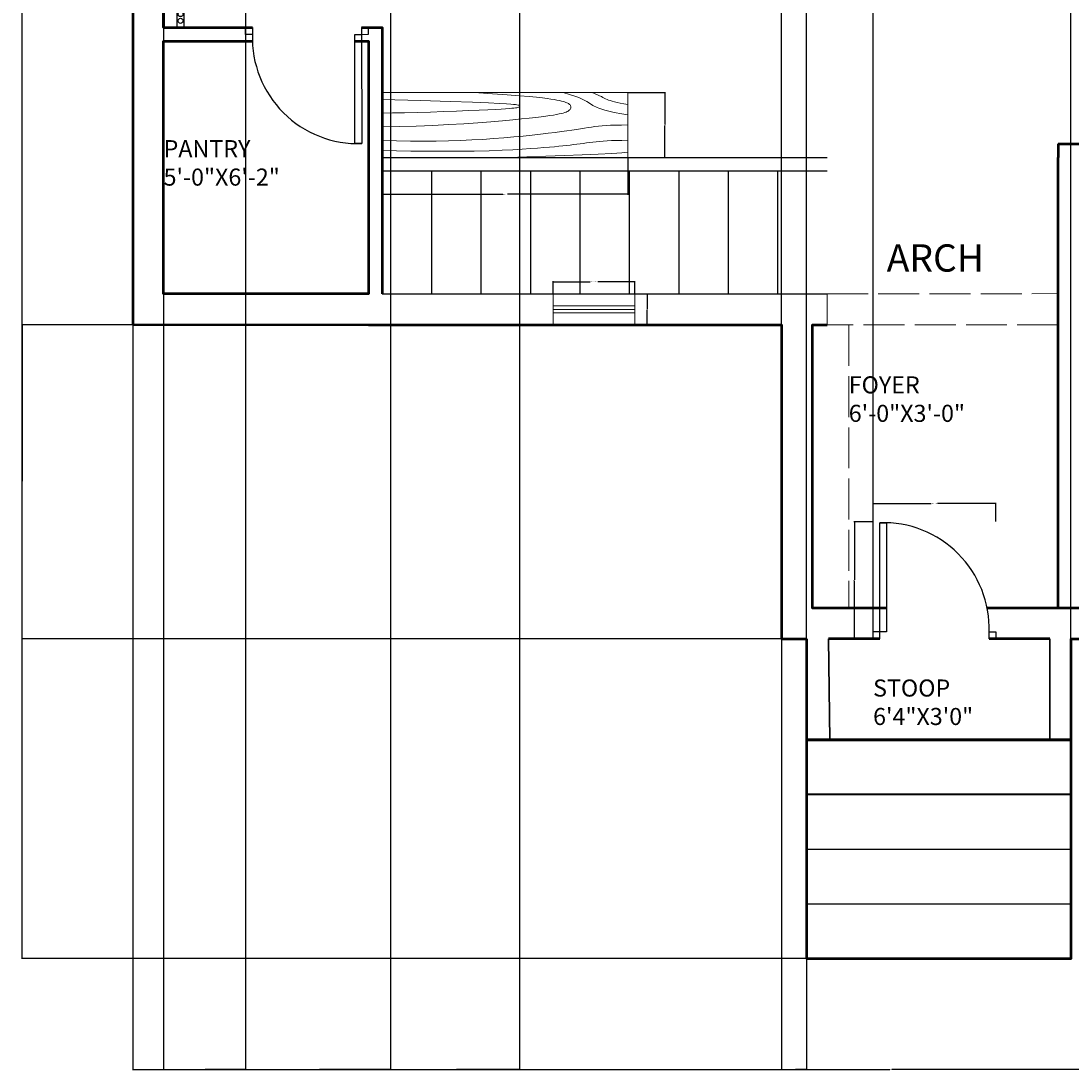
# Model space of a CAD drawing. Units: inches. Extents: x 821 to 2399, y 74 to 823.
# Tile 1 of 13: x 821 to 1128, y 74 to 381. Entities that reach past the tile are written whole.
import ezdxf

# ---------------------------------------------------------------- set-up
doc = ezdxf.new("R2010")
doc.units = ezdxf.units.IN
doc.header["$MEASUREMENT"] = 0
doc.linetypes.add('ACAD_ISO02W100', pattern=[15, 12, -3])
doc.layers.get('0').update_dxf_attribs({"lineweight": 53})
for name, color, linetype, lineweight in [('A-ANNO-DIMS', 2, 'Continuous', 18), ('A-ANNO-TEXT', 7, 'Continuous', 18), ('A-AREA-IDEN', 7, 'Continuous', 18), ('A-DOOR', 4, 'Continuous', 25), ('A-EQPM', 9, 'Continuous', 25), ('A-FLOR', 7, 'Continuous', 30), ('A-FLOR-CASE', 9, 'Continuous', 25), ('A-FLOR-STRS', 7, 'Continuous', 25), ('A-FURN', 8, 'Continuous', 18), ('A-GLAZ', 4, 'Continuous', 18), ('A-WALL-OVHD', 8, 'ACAD_ISO02W100', 18), ('WALLS', 7, 'Continuous', 50)]:
    doc.layers.add(name, color=color, linetype=linetype, lineweight=lineweight)
doc.styles.get("Standard").update_dxf_attribs({"font": 'arial.ttf'})
doc.dimstyles.get("Standard").update_dxf_attribs({"dimtxt": 0.18, "dimasz": 0.18, "dimexe": 0.18, "dimexo": 0.0625, "dimgap": 0.09, "dimtad": 0, "dimtih": 1, "dimtoh": 1, "dimdec": 4, "dimzin": 0, "dimdsep": 46, "dimtxsty": 'Standard', "dimcen": 0.09, "dimadec": 0, "dimazin": 0, "dimtfac": 1, "dimtdec": 4, "dimtofl": 0, "dimtmove": 0, "dimatfit": 3, "dimfxl": 1, "dimtolj": 1, "dimtzin": 0, "dimarcsym": 0})

# ---------------------------------------------------------------- blocks, each defined once
blk = doc.blocks.new('Hutch - 19 x 72 in.')
for p, q in [((0, -19), (0, 0)), ((0, 0), (71.999994, 0)), ((71.999994, 0), (71.999994, -19)), ((71.999994, -19), (0, -19))]:
    blk.add_line(p, q)
for points in [[(26.99999, 0), (32.30411, -0.35238), (36.66731, -0.66276), (40.20336, -0.93603), (43.02603, -1.17708), (45.2491, -1.39079), (46.98632, -1.58203), (48.35147, -1.7557), (49.45833, -1.91667), (50.40388, -2.06917), (51.21809, -2.21484), (51.91414, -2.35465), (52.5052, -2.48958), (53.00447, -2.6206), (53.42512, -2.7487), (53.78035, -2.87484), (54.08333, -3), (54.34537, -3.12516), (54.57031, -3.2513), (54.76008, -3.37939), (54.91666, -3.51042), (55.04198, -3.64534), (55.13801, -3.78516), (55.2067, -3.93083), (55.24999, -4.08333), (55.26904, -4.24316), (55.26171, -4.40885), (55.22509, -4.57845), (55.15624, -4.75), (55.05224, -4.92155), (54.91015, -5.09115), (54.72704, -5.25684), (54.49999, -5.41667), (54.22493, -5.56934), (53.89322, -5.71615), (53.49511, -5.85905), (53.02083, -6), (52.4606, -6.14095), (51.80468, -6.28385), (51.04329, -6.43066), (50.16666, -6.58333), (49.16007, -6.74381), (47.98892, -6.91406), (46.61368, -7.09603), (44.99478, -7.29167), (43.09268, -7.50293), (40.86783, -7.73177), (38.28067, -7.98014), (35.29166, -8.25), (31.87654, -8.54053), (28.07226, -8.83984), (23.93107, -9.1333), (19.5052, -9.40625), (14.84692, -9.64404), (10.00846, -9.83203), (5.04207, -9.95557), (0, -10)], [(52.99999, 0), (54.87133, -0.53955), (56.39257, -1.03516), (57.61205, -1.48975), (58.57812, -1.90625), (59.3391, -2.2876), (59.94335, -2.63672), (60.4392, -2.95654), (60.87499, -3.25), (61.29247, -3.52002), (61.70702, -3.76953), (62.12743, -4.00146), (62.56249, -4.21875), (63.02099, -4.42432), (63.51171, -4.62109), (64.04345, -4.81201), (64.62499, -5), (65.26489, -5.1875), (65.9707, -5.375), (66.74975, -5.5625), (67.60937, -5.75), (68.55688, -5.9375), (69.5996, -6.125), (70.744867, -6.3125), (71.999994, -6.5)], [(61.49999, 0), (62.35961, -0.35254), (63.08007, -0.66406), (63.68627, -0.94043), (64.20312, -1.1875), (64.65551, -1.41113), (65.06835, -1.61719), (65.46655, -1.81152), (65.87499, -2), (66.31762, -2.1875), (66.81445, -2.375), (67.38452, -2.5625), (68.04687, -2.75), (68.82055, -2.9375), (69.7246, -3.125), (70.77807, -3.3125), (71.999994, -3.5)], [(0, -2), (11.2006, -2.34123), (19.90169, -2.62044), (26.43969, -2.84595), (31.15103, -3.02604), (34.37214, -3.16903), (36.43945, -3.2832), (37.68936, -3.37687), (38.45833, -3.45833), (39.02937, -3.53459), (39.472, -3.60742), (39.80232, -3.67733), (40.03645, -3.74479), (40.1905, -3.8103), (40.28059, -3.87435), (40.32283, -3.93742), (40.33333, -4), (40.32405, -4.0625), (40.29036, -4.125), (40.22346, -4.1875), (40.11458, -4.25), (39.95491, -4.3125), (39.73567, -4.375), (39.44807, -4.4375), (39.08333, -4.5), (38.62491, -4.56282), (38.02538, -4.6276), (37.22957, -4.69629), (36.18228, -4.77083), (34.82836, -4.85319), (33.11262, -4.94531), (30.97989, -5.04915), (28.37499, -5.16667), (25.27416, -5.29818), (21.77929, -5.4375), (18.02368, -5.57682), (14.14062, -5.70833), (10.26342, -5.82422), (6.52539, -5.91667), (3.05981, -5.97786), (0, -6)], [(71.999994, -9.5), (70.071934, -9.51147), (68.38801, -9.54492), (66.91113, -9.59888), (65.60416, -9.67187), (64.43001, -9.76245), (63.35156, -9.86914), (62.3317, -9.99048), (61.33333, -10.125), (60.32128, -10.27157), (59.26822, -10.43034), (58.14876, -10.60181), (56.93749, -10.78646), (55.60904, -10.98478), (54.13801, -11.19726), (52.49902, -11.4244), (50.66666, -11.66667), (48.62239, -11.92358), (46.37499, -12.19075), (43.9401, -12.46281), (41.33333, -12.73437), (38.57031, -13.00008), (35.66666, -13.25456), (32.63801, -13.49243), (29.49999, -13.70833), (26.26367, -13.89689), (22.92187, -14.05273), (19.46289, -14.17049), (15.875, -14.24479), (12.14648, -14.27026), (8.26562, -14.24154), (4.2207, -14.15324), (0, -14)], [(0, -17), (8.37556, -17.14274), (15.58268, -17.20443), (21.74194, -17.19775), (26.97395, -17.13542), (31.39933, -17.03011), (35.13866, -16.89453), (38.31257, -16.74137), (41.04166, -16.58333), (43.4322, -16.43083), (45.5332, -16.28516), (47.37931, -16.14534), (49.0052, -16.01042), (50.44555, -15.87939), (51.73502, -15.7513), (52.90828, -15.62516), (53.99999, -15.5), (55.04044, -15.37508), (56.04231, -15.25065), (57.01391, -15.1272), (57.96353, -15.00521), (58.89949, -14.88517), (59.83007, -14.76758), (60.76358, -14.65291), (61.70833, -14.54167), (62.6752, -14.43465), (63.68554, -14.33398), (64.76326, -14.24211), (65.93229, -14.16146), (67.21655, -14.09448), (68.63997, -14.04362), (70.226475, -14.01131), (71.999994, -14)], [(36.99999, -19), (42.40038, -18.8125), (47.95312, -18.625), (53.43554, -18.4375), (58.62499, -18.25), (63.29882, -18.0625), (67.23437, -17.875), (70.208978, -17.6875), (71.999994, -17.5)]]:
    blk.add_lwpolyline(points)
blk = doc.blocks.new('Range Hood - 30 in front')
blk.add_line((0, -4), (30.0001, -4))
for points in [[(0, -6), (0, 0), (30.0001, 0), (30.0001, -6)], [(23, -5.75), (23, -4.25), (29, -4.25), (29, -5.75)]]:
    blk.add_lwpolyline(points, close=True)
for centre in [(2, -5), (4, -5)]:
    blk.add_circle(centre, 0.75)
blk = doc.blocks.new('DOOR-SWING-32IN')
for p, q in [((0, 0), (2, 0)), ((34, 0), (36, 0))]:
    blk.add_line(p, q)
blk.add_lwpolyline([(34, 2, 0.433232), (2, 34), (4, 34), (4, 2), (2, 2), (2, 34)], format="xyb")
for points in [[(0, 0), (2, 0), (2, 2), (0, 2)], [(36, 0), (34, 0), (34, 2), (36, 2)]]:
    blk.add_lwpolyline(points, close=True)
blk = doc.blocks.new('WIN-24IN')
for p, q in [((3.5, 24), (3.5, 0)), ((4.5, 24), (4.5, 0)), ((5.5, 24), (5.5, 0))]:
    blk.add_line(p, q)
blk.add_lwpolyline([(0, 24), (9, 24), (9, 0), (0, 0)], close=True)
blk = doc.blocks.new('*D28')
at = {"layer": 'A-ANNO-DIMS', "color": 0, "lineweight": -2, "transparency": 16777216}
for p, q in [((1070.14, 234.86), (1070.14, 240.38)), ((1070.32, 240.2), (1087.2, 240.2)), ((1105.96, 240.2), (1089.07, 240.2)), ((1106.14, 234.86), (1106.14, 240.38))]:
    blk.add_line(p, q, dxfattribs=at)
at = {"layer": 'A-ANNO-DIMS', "color": 0, "lineweight": 50, "transparency": 16777216}
for points in [[(1070.32, 240.23), (1070.32, 240.17), (1070.14, 240.2)], [(1105.96, 240.23), (1105.96, 240.17), (1106.14, 240.2)]]:
    blk.add_solid(points, dxfattribs=at)
at = {"layer": 'Defpoints', "color": 0, "lineweight": 50, "transparency": 16777216}
for p in [(1106.14, 240.2), (1070.14, 234.8), (1106.14, 234.8)]:
    blk.add_point(p, dxfattribs=at)
at = {"layer": 'A-ANNO-DIMS', "color": 0, "transparency": 16777216, "insert": (1088.14, 240.2), "char_height": 0.18, "attachment_point": 5}
blk.add_mtext('\\A1;DOOR 36 TYP.', dxfattribs=at)
blk = doc.blocks.new('*D29')
at = {"layer": 'A-ANNO-DIMS', "color": 0, "lineweight": -2, "transparency": 16777216}
for p, q in [((1070.07, 234.8), (1064.56, 234.8)), ((1064.74, 234.62), (1064.74, 217.84)), ((1064.74, 200.7), (1064.74, 217.48)), ((1070.07, 200.52), (1064.56, 200.52))]:
    blk.add_line(p, q, dxfattribs=at)
at = {"layer": 'A-ANNO-DIMS', "color": 0, "lineweight": 50, "transparency": 16777216}
for points in [[(1064.71, 234.62), (1064.77, 234.62), (1064.74, 234.8)], [(1064.71, 200.7), (1064.77, 200.7), (1064.74, 200.52)]]:
    blk.add_solid(points, dxfattribs=at)
at = {"layer": 'Defpoints', "color": 0, "lineweight": 50, "transparency": 16777216}
for p in [(1064.74, 234.8), (1070.14, 234.8), (1070.14, 200.52)]:
    blk.add_point(p, dxfattribs=at)
at = {"layer": 'A-ANNO-DIMS', "color": 0, "transparency": 16777216, "insert": (1064.74, 217.66), "char_height": 0.18, "attachment_point": 5}
blk.add_mtext('\\A1;34 TYP.', dxfattribs=at)
blk = doc.blocks.new('*D32')
at = {"layer": 'A-ANNO-DIMS', "color": 0, "lineweight": -2, "transparency": 16777216}
for p, q in [((976.43, 301.58), (976.43, 305.3)), ((976.61, 305.12), (987.31, 305.12)), ((1000.25, 305.12), (989.54, 305.12)), ((1000.43, 301.58), (1000.43, 305.3))]:
    blk.add_line(p, q, dxfattribs=at)
at = {"layer": 'A-ANNO-DIMS', "color": 0, "lineweight": 50, "transparency": 16777216}
for points in [[(976.61, 305.15), (976.61, 305.09), (976.43, 305.12)], [(1000.25, 305.15), (1000.25, 305.09), (1000.43, 305.12)]]:
    blk.add_solid(points, dxfattribs=at)
at = {"layer": 'Defpoints', "color": 0, "lineweight": 50, "transparency": 16777216}
for p in [(1000.43, 305.12), (976.43, 301.52), (1000.43, 301.52)]:
    blk.add_point(p, dxfattribs=at)
at = {"layer": 'A-ANNO-DIMS', "color": 0, "transparency": 16777216, "insert": (988.43, 305.12), "char_height": 0.18, "attachment_point": 5}
blk.add_mtext('\\A1;WINDOW 24 TYP.', dxfattribs=at)
blk = doc.blocks.new('*D33')
at = {"layer": 'A-ANNO-DIMS', "color": 0, "lineweight": -2, "transparency": 16777216}
for p, q in [((1000.49, 301.52), (1004.21, 301.52)), ((1004.03, 301.34), (1004.03, 297.2)), ((1004.03, 292.7), (1004.03, 296.84)), ((1000.49, 292.52), (1004.21, 292.52))]:
    blk.add_line(p, q, dxfattribs=at)
at = {"layer": 'A-ANNO-DIMS', "color": 0, "lineweight": 50, "transparency": 16777216}
for points in [[(1004, 301.34), (1004.06, 301.34), (1004.03, 301.52)], [(1004, 292.7), (1004.06, 292.7), (1004.03, 292.52)]]:
    blk.add_solid(points, dxfattribs=at)
at = {"layer": 'Defpoints', "color": 0, "lineweight": 50, "transparency": 16777216}
for p in [(1000.43, 301.52), (1000.43, 292.52), (1004.03, 292.52)]:
    blk.add_point(p, dxfattribs=at)
at = {"layer": 'A-ANNO-DIMS', "color": 0, "transparency": 16777216, "insert": (1004.03, 297.02), "char_height": 0.18, "attachment_point": 5}
blk.add_mtext('\\A1;9 TYP.', dxfattribs=at)
blk = doc.blocks.new('*D46')
at = {"layer": 'A-ANNO-DIMS', "color": 0, "lineweight": -2, "transparency": 16777216}
for p, q in [((926.37, 341.46), (926.37, 330.54)), ((998.37, 341.46), (998.37, 330.54)), ((926.55, 330.72), (961.69, 330.72)), ((998.19, 330.72), (963.06, 330.72))]:
    blk.add_line(p, q, dxfattribs=at)
at = {"layer": 'A-ANNO-DIMS', "color": 0, "lineweight": 50, "transparency": 16777216}
for points in [[(926.55, 330.75), (926.55, 330.69), (926.37, 330.72)], [(998.19, 330.75), (998.19, 330.69), (998.37, 330.72)]]:
    blk.add_solid(points, dxfattribs=at)
at = {"layer": 'Defpoints', "color": 0, "lineweight": 50, "transparency": 16777216}
for p in [(926.37, 341.52), (998.37, 341.52), (998.37, 330.72)]:
    blk.add_point(p, dxfattribs=at)
at = {"layer": 'A-ANNO-DIMS', "color": 0, "transparency": 16777216, "insert": (962.37, 330.72), "char_height": 0.18, "attachment_point": 5}
blk.add_mtext('\\A1;HUTCH 72', dxfattribs=at)
blk = doc.blocks.new('*D47')
at = {"layer": 'A-ANNO-DIMS', "color": 0, "lineweight": -2, "transparency": 16777216}
for p, q in [((998.44, 360.52), (1009.35, 360.52)), ((1009.17, 360.34), (1009.17, 351.2)), ((1009.17, 341.7), (1009.17, 350.84)), ((998.44, 341.52), (1009.35, 341.52))]:
    blk.add_line(p, q, dxfattribs=at)
at = {"layer": 'A-ANNO-DIMS', "color": 0, "lineweight": 50, "transparency": 16777216}
for points in [[(1009.14, 360.34), (1009.2, 360.34), (1009.17, 360.52)], [(1009.14, 341.7), (1009.2, 341.7), (1009.17, 341.52)]]:
    blk.add_solid(points, dxfattribs=at)
at = {"layer": 'Defpoints', "color": 0, "lineweight": 50, "transparency": 16777216}
for p in [(998.37, 360.52), (1009.17, 360.52), (998.37, 341.52)]:
    blk.add_point(p, dxfattribs=at)
at = {"layer": 'A-ANNO-DIMS', "color": 0, "transparency": 16777216, "insert": (1009.17, 351.02), "char_height": 0.18, "attachment_point": 5}
blk.add_mtext('\\A1;19', dxfattribs=at)
blk = doc.blocks.new('*D78')
at = {"layer": 'A-ANNO-DIMS', "color": 0, "lineweight": -2, "transparency": 16777216}
for p, q in [((853.37, 292.49), (853.37, 74.23)), ((1297.37, 200.46), (1297.37, 74.23)), ((853.55, 74.41), (1075.08, 74.41)), ((1297.19, 74.41), (1075.67, 74.41))]:
    blk.add_line(p, q, dxfattribs=at)
at = {"layer": 'A-ANNO-DIMS', "color": 0, "lineweight": 50, "transparency": 16777216}
for points in [[(853.55, 74.44), (853.55, 74.38), (853.37, 74.41)], [(1297.19, 74.44), (1297.19, 74.38), (1297.37, 74.41)]]:
    blk.add_solid(points, dxfattribs=at)
at = {"layer": 'Defpoints', "color": 0, "lineweight": 50, "transparency": 16777216}
for p in [(853.37, 292.55), (1297.37, 200.52), (1297.37, 74.41)]:
    blk.add_point(p, dxfattribs=at)
at = {"layer": 'A-ANNO-DIMS', "color": 0, "transparency": 16777216, "insert": (1075.37, 74.41), "char_height": 0.18, "attachment_point": 5}
blk.add_mtext('\\A1;444', dxfattribs=at)
blk = doc.blocks.new('*D80')
at = {"layer": 'A-ANNO-DIMS', "color": 0, "lineweight": -2, "transparency": 16777216}
for p, q in [((999.33, 754.12), (820.74, 754.12)), ((820.92, 753.94), (820.92, 430.67)), ((820.92, 107.04), (820.92, 430.31)), ((1050.58, 106.86), (820.74, 106.86))]:
    blk.add_line(p, q, dxfattribs=at)
at = {"layer": 'A-ANNO-DIMS', "color": 0, "lineweight": 50, "transparency": 16777216}
for points in [[(820.89, 753.94), (820.95, 753.94), (820.92, 754.12)], [(820.89, 107.04), (820.95, 107.04), (820.92, 106.86)]]:
    blk.add_solid(points, dxfattribs=at)
at = {"layer": 'Defpoints', "color": 0, "lineweight": 50, "transparency": 16777216}
for p in [(999.39, 754.12), (820.92, 106.86), (1050.64, 106.86)]:
    blk.add_point(p, dxfattribs=at)
at = {"layer": 'A-ANNO-DIMS', "color": 0, "transparency": 16777216, "insert": (820.92, 430.49), "char_height": 0.18, "attachment_point": 5}
blk.add_mtext('\\A1;647.3', dxfattribs=at)
blk = doc.blocks.new('*D81')
at = {"layer": 'A-ANNO-DIMS', "color": 0, "lineweight": -2, "transparency": 16777216}
for p, q in [((853.37, 292.61), (853.37, 786.75)), ((853.55, 786.57), (948.09, 786.57)), ((1043.19, 786.57), (948.65, 786.57)), ((1043.37, 292.58), (1043.37, 786.75))]:
    blk.add_line(p, q, dxfattribs=at)
at = {"layer": 'A-ANNO-DIMS', "color": 0, "lineweight": 50, "transparency": 16777216}
for points in [[(853.55, 786.6), (853.55, 786.54), (853.37, 786.57)], [(1043.19, 786.6), (1043.19, 786.54), (1043.37, 786.57)]]:
    blk.add_solid(points, dxfattribs=at)
at = {"layer": 'Defpoints', "color": 0, "lineweight": 50, "transparency": 16777216}
for p in [(1043.37, 786.57), (853.37, 292.55), (1043.37, 292.52)]:
    blk.add_point(p, dxfattribs=at)
at = {"layer": 'A-ANNO-DIMS', "color": 0, "transparency": 16777216, "insert": (948.37, 786.57), "char_height": 0.18, "attachment_point": 5}
blk.add_mtext('\\A1;190', dxfattribs=at)
blk = doc.blocks.new('*D82')
at = {"layer": 'A-ANNO-DIMS', "color": 0, "lineweight": -2, "transparency": 16777216}
for p, q in [((1043.31, 292.52), (820.74, 292.52)), ((820.92, 292.34), (820.92, 246.7)), ((820.92, 200.7), (820.92, 246.34)), ((1043.31, 200.52), (820.74, 200.52))]:
    blk.add_line(p, q, dxfattribs=at)
at = {"layer": 'A-ANNO-DIMS', "color": 0, "lineweight": 50, "transparency": 16777216}
for points in [[(820.89, 292.34), (820.95, 292.34), (820.92, 292.52)], [(820.89, 200.7), (820.95, 200.7), (820.92, 200.52)]]:
    blk.add_solid(points, dxfattribs=at)
at = {"layer": 'Defpoints', "color": 0, "lineweight": 50, "transparency": 16777216}
for p in [(1043.37, 292.52), (820.92, 200.52), (1043.37, 200.52)]:
    blk.add_point(p, dxfattribs=at)
at = {"layer": 'A-ANNO-DIMS', "color": 0, "transparency": 16777216, "insert": (820.92, 246.52), "char_height": 0.18, "attachment_point": 5}
blk.add_mtext('\\A1;92', dxfattribs=at)
blk = doc.blocks.new('*D89')
at = {"layer": 'A-ANNO-DIMS', "color": 0, "lineweight": -2, "transparency": 16777216}
for p, q in [((1050.64, 106.93), (1050.64, 786.75)), ((1050.82, 786.57), (1088.99, 786.57)), ((1127.94, 786.57), (1089.78, 786.57)), ((1128.12, 106.93), (1128.12, 786.75))]:
    blk.add_line(p, q, dxfattribs=at)
at = {"layer": 'A-ANNO-DIMS', "color": 0, "lineweight": 50, "transparency": 16777216}
for points in [[(1050.82, 786.6), (1050.82, 786.54), (1050.64, 786.57)], [(1127.94, 786.6), (1127.94, 786.54), (1128.12, 786.57)]]:
    blk.add_solid(points, dxfattribs=at)
at = {"layer": 'Defpoints', "color": 0, "lineweight": 50, "transparency": 16777216}
for p in [(1128.12, 786.57), (1050.64, 106.86), (1128.12, 106.86)]:
    blk.add_point(p, dxfattribs=at)
at = {"layer": 'A-ANNO-DIMS', "color": 0, "transparency": 16777216, "insert": (1089.38, 786.57), "char_height": 0.18, "attachment_point": 5}
blk.add_mtext('\\A1;77.48', dxfattribs=at)
blk = doc.blocks.new('*D90')
at = {"layer": 'A-ANNO-DIMS', "color": 0, "lineweight": -2, "transparency": 16777216}
for p, q in [((1043.37, 200.46), (1043.37, 74.23)), ((1050.64, 200.46), (1050.64, 74.23)), ((1043.55, 74.41), (1046.61, 74.41)), ((1050.46, 74.41), (1047.4, 74.41))]:
    blk.add_line(p, q, dxfattribs=at)
at = {"layer": 'A-ANNO-DIMS', "color": 0, "lineweight": 50, "transparency": 16777216}
for points in [[(1043.55, 74.44), (1043.55, 74.38), (1043.37, 74.41)], [(1050.46, 74.44), (1050.46, 74.38), (1050.64, 74.41)]]:
    blk.add_solid(points, dxfattribs=at)
at = {"layer": 'Defpoints', "color": 0, "lineweight": 50, "transparency": 16777216}
for p in [(1043.37, 200.52), (1050.64, 200.52), (1050.64, 74.41)]:
    blk.add_point(p, dxfattribs=at)
at = {"layer": 'A-ANNO-DIMS', "color": 0, "transparency": 16777216, "insert": (1047.01, 74.41), "char_height": 0.18, "attachment_point": 5}
blk.add_mtext('\\A1;7.268', dxfattribs=at)
blk = doc.blocks.new('*D91')
at = {"layer": 'A-ANNO-DIMS', "color": 0, "lineweight": -2, "transparency": 16777216}
for p, q in [((1043.37, 200.58), (1043.37, 786.75)), ((1043.55, 786.57), (1056.29, 786.57)), ((1069.96, 786.57), (1057.22, 786.57)), ((1070.14, 200.58), (1070.14, 786.75))]:
    blk.add_line(p, q, dxfattribs=at)
at = {"layer": 'A-ANNO-DIMS', "color": 0, "lineweight": 50, "transparency": 16777216}
for points in [[(1043.55, 786.6), (1043.55, 786.54), (1043.37, 786.57)], [(1069.96, 786.6), (1069.96, 786.54), (1070.14, 786.57)]]:
    blk.add_solid(points, dxfattribs=at)
at = {"layer": 'Defpoints', "color": 0, "lineweight": 50, "transparency": 16777216}
for p in [(1070.14, 786.57), (1043.37, 200.52), (1070.14, 200.52)]:
    blk.add_point(p, dxfattribs=at)
at = {"layer": 'A-ANNO-DIMS', "color": 0, "transparency": 16777216, "insert": (1056.75, 786.57), "char_height": 0.18, "attachment_point": 5}
blk.add_mtext('\\A1;26.763', dxfattribs=at)
blk = doc.blocks.new('*D100')
at = {"layer": 'A-ANNO-DIMS', "color": 0, "lineweight": -2, "transparency": 16777216}
for p, q in [((862.37, 379.46), (862.37, 74.23)), ((886.37, 379.46), (886.37, 74.23)), ((862.55, 74.41), (874.15, 74.41)), ((886.19, 74.41), (874.59, 74.41))]:
    blk.add_line(p, q, dxfattribs=at)
at = {"layer": 'A-ANNO-DIMS', "color": 0, "lineweight": 50, "transparency": 16777216}
for points in [[(862.55, 74.44), (862.55, 74.38), (862.37, 74.41)], [(886.19, 74.44), (886.19, 74.38), (886.37, 74.41)]]:
    blk.add_solid(points, dxfattribs=at)
at = {"layer": 'Defpoints', "color": 0, "lineweight": 50, "transparency": 16777216}
for p in [(862.37, 379.52), (886.37, 379.52), (886.37, 74.41)]:
    blk.add_point(p, dxfattribs=at)
at = {"layer": 'A-ANNO-DIMS', "color": 0, "transparency": 16777216, "insert": (874.37, 74.41), "char_height": 0.18, "attachment_point": 5}
blk.add_mtext('\\A1;24', dxfattribs=at)
blk = doc.blocks.new('*D101')
at = {"layer": 'A-ANNO-DIMS', "color": 0, "lineweight": -2, "transparency": 16777216}
for p, q in [((928.85, 427.27), (928.85, 74.23)), ((886.37, 379.46), (886.37, 74.23)), ((886.55, 74.41), (907.21, 74.41)), ((928.67, 74.41), (908.01, 74.41))]:
    blk.add_line(p, q, dxfattribs=at)
at = {"layer": 'A-ANNO-DIMS', "color": 0, "lineweight": 50, "transparency": 16777216}
for points in [[(886.55, 74.44), (886.55, 74.38), (886.37, 74.41)], [(928.67, 74.44), (928.67, 74.38), (928.85, 74.41)]]:
    blk.add_solid(points, dxfattribs=at)
at = {"layer": 'Defpoints', "color": 0, "lineweight": 50, "transparency": 16777216}
for p in [(928.85, 427.33), (886.37, 379.52), (928.85, 74.41)]:
    blk.add_point(p, dxfattribs=at)
at = {"layer": 'A-ANNO-DIMS', "color": 0, "transparency": 16777216, "insert": (907.61, 74.41), "char_height": 0.18, "attachment_point": 5}
blk.add_mtext('\\A1;42.48', dxfattribs=at)
blk = doc.blocks.new('*D102')
at = {"layer": 'A-ANNO-DIMS', "color": 0, "lineweight": -2, "transparency": 16777216}
for p, q in [((928.85, 427.27), (928.85, 74.23)), ((966.61, 427.27), (966.61, 74.23)), ((929.03, 74.41), (947.34, 74.41)), ((966.43, 74.41), (948.12, 74.41))]:
    blk.add_line(p, q, dxfattribs=at)
at = {"layer": 'A-ANNO-DIMS', "color": 0, "lineweight": 50, "transparency": 16777216}
for points in [[(929.03, 74.44), (929.03, 74.38), (928.85, 74.41)], [(966.43, 74.44), (966.43, 74.38), (966.61, 74.41)]]:
    blk.add_solid(points, dxfattribs=at)
at = {"layer": 'Defpoints', "color": 0, "lineweight": 50, "transparency": 16777216}
for p in [(928.85, 427.33), (966.61, 427.33), (966.61, 74.41)]:
    blk.add_point(p, dxfattribs=at)
at = {"layer": 'A-ANNO-DIMS', "color": 0, "transparency": 16777216, "insert": (947.73, 74.41), "char_height": 0.18, "attachment_point": 5}
blk.add_mtext('\\A1;37.76', dxfattribs=at)

msp = doc.modelspace()

# ---------------------------------------------------------------- linework, layer by layer
at = {"layer": 'A-FLOR'}
for p, q in [((1057.4756, 170.9407), (1057.0959, 200.5195)), ((1121.9086, 170.9407), (1121.9086, 200.5195)), ((1050.641, 170.9407), (1057.4756, 170.9407))]:
    msp.add_line(p, q, dxfattribs=at)
at = {"layer": 'A-FLOR-CASE'}
msp.add_line((886.3735, 589.5195), (886.3735, 379.5195), dxfattribs=at)
at = {"layer": 'A-FLOR-STRS'}
for p, q in [((926.3735, 341.5195), (1056.6808, 341.5195)), ((940.8521, 337.5195), (940.8521, 301.5195)), ((955.3306, 337.5195), (955.3306, 301.5195)), ((969.8092, 337.5195), (969.8092, 301.5195)), ((984.2878, 337.5195), (984.2878, 301.5195)), ((998.7664, 337.5195), (998.7664, 301.5195)), ((1013.245, 337.5195), (1013.245, 301.5195)), ((1027.7236, 337.5195), (1027.7236, 301.5195)), ((1042.2022, 337.5195), (1042.2022, 301.5195)), ((1050.641, 155.1305), (1128.124, 155.1305)), ((1050.641, 154.9216), (1128.124, 154.9216)), ((1050.641, 138.9026), (1128.124, 138.9026)), ((1050.641, 122.8835), (1128.124, 122.8835))]:
    msp.add_line(p, q, dxfattribs=at)
msp.add_lwpolyline([(1056.6808, 337.5195), (926.3735, 337.5195), (926.3735, 301.5195), (1056.6808, 301.5195)], dxfattribs=at)
at = {"layer": 'A-WALL-OVHD'}
msp.add_line((1063.0337, 292.458), (1063.0318, 209.5195), dxfattribs=at)
msp.add_lwpolyline([(1124.3735, 292.446), (1056.6808, 292.5195), (1056.6808, 301.5195), (1124.3735, 301.616)], dxfattribs=at)
at = {"layer": 'WALLS'}
for p, q in [((1124.3735, 345.5195), (1159.7172, 345.5195)), ((1124.3735, 345.5195), (1124.3735, 341.5195)), ((1124.3735, 209.5195), (1124.3735, 341.5195)), ((922.3762, 305.5195), (922.3735, 305.5195)), ((918.3735, 301.5222), (918.3735, 301.5195)), ((922.3673, 301.5195), (922.3735, 301.5195)), ((1072.1365, 200.5195), (1057.0959, 200.5195)), ((1121.9086, 200.5195), (1104.1365, 200.5195))]:
    msp.add_line(p, q, dxfattribs=at)
msp.add_lwpolyline([(1050.641, 200.5195), (1050.641, 170.9407), (1121.9086, 170.9407), (1128.124, 170.9407), (1050.641, 170.9407), (1050.641, 106.8645), (1128.124, 106.8645), (1128.124, 170.9407), (1128.124, 200.5195), (1288.3735, 200.5195), (1297.3735, 200.5195), (1297.3735, 598.5195), (853.3735, 598.5195), (853.3735, 292.549), (922.3673, 292.5195), (1043.3735, 292.5195), (1043.3735, 209.5195), (1043.3735, 200.5195)], close=True, dxfattribs=at)
for points in [[(862.3735, 379.5195), (862.3735, 589.5195), (862.3735, 379.5195), (888.3735, 379.5195)], [(920.3735, 379.5195), (926.3735, 379.5195), (926.3735, 301.5195)], [(918.3788, 375.5195), (922.3735, 375.5195), (922.3735, 301.5195), (862.3735, 301.5605), (862.3735, 375.5195), (888.3788, 375.5195)], [(1191.7172, 341.5195), (1288.3735, 341.5195), (1288.3735, 209.5195), (1103.5667, 209.5195)], [(1074.1365, 209.5195), (1052.3735, 209.5195), (1052.3735, 292.5195), (1056.6808, 292.5195)]]:
    msp.add_lwpolyline(points, dxfattribs=at)

# ---------------------------------------------------------------- block references
at = {"layer": 'A-DOOR', "rotation": 180.0755959281295}
msp.add_blockref('DOOR-SWING-32IN', (922.3739, 379.5674), dxfattribs=at)
at = {"layer": 'A-DOOR'}
msp.add_blockref('DOOR-SWING-32IN', (1070.136, 200.519), dxfattribs=at)
at = {"layer": 'A-EQPM', "rotation": 90}
msp.add_blockref('Range Hood - 30 in front', (862.3528, 379.5195), dxfattribs=at)
at = {"layer": 'A-FURN'}
msp.add_blockref('Hutch - 19 x 72 in.', (926.3735, 360.5195), dxfattribs=at)
at = {"layer": 'A-GLAZ', "rotation": 269.9999999999995}
msp.add_blockref('WIN-24IN', (976.4247, 301.5199), dxfattribs=at)

# ---------------------------------------------------------------- texts
at = {"layer": 'A-ANNO-TEXT', "insert": (1074.1559, 316.0646), "char_height": 8, "attachment_point": 1}
msp.add_mtext_dynamic_manual_height_columns('ARCH', width=40.787909, gutter_width=1, heights=[0], dxfattribs=at)
at = {"layer": 'A-AREA-IDEN', "char_height": 5, "attachment_point": 1}
for s, width, insert in [('PANTRY\\P5\'-0"X6\'-2"', 60, (862.3735, 346.5855)), ('FOYER\\P6\'-0"X3\'-0"', 61.340069, (1063.0334, 277.3957)), ('STOOP\\P6\'4"X3\'0"', 43.932247, (1070.1619, 188.6098))]:
    msp.add_mtext_dynamic_manual_height_columns(s, width=width, gutter_width=1, heights=[0], dxfattribs=dict(at, insert=insert))

# ---------------------------------------------------------------- dimensions: what is measured, and where the dimension line sits
at = {"layer": 'A-ANNO-DIMS'}
for base, p1, p2, override, picture, middle in [((1043.3735, 786.5664), (853.3735, 292.549), (1043.3735, 292.5195), {"dimdec": 0, "dimlfac": 1, "dimrnd": 0, "dimzin": 0, "dimdsep": 46, "dimlunit": 2}, '*D81', (948.3735, 786.5664)), ((1070.1365, 786.5664), (1043.3735, 200.5195), (1070.1365, 200.5195), {"dimdec": 3, "dimlfac": 1, "dimrnd": 0, "dimzin": 0, "dimdsep": 46, "dimlunit": 2}, '*D91', (1056.755, 786.5664)), ((1128.124, 786.5664), (1050.641, 106.8645), (1128.124, 106.8645), {"dimdec": 2, "dimlfac": 1, "dimrnd": 0, "dimzin": 0, "dimdsep": 46, "dimlunit": 2}, '*D89', (1089.3825, 786.5664)), ((928.8511, 74.4145), (886.3735, 379.5195), (928.8511, 427.3294), {"dimdec": 2, "dimlfac": 1, "dimrnd": 0, "dimzin": 0, "dimdsep": 46, "dimlunit": 2}, '*D101', (907.6123, 74.4145)), ((966.6107, 74.4145), (928.8511, 427.3294), (966.6107, 427.3294), {"dimdec": 2, "dimlfac": 1, "dimrnd": 0, "dimzin": 0, "dimdsep": 46, "dimlunit": 2}, '*D102', (947.7309, 74.4145)), ((886.3735, 74.4145), (862.3735, 379.5195), (886.3735, 379.5195), {"dimdec": 0, "dimlfac": 1, "dimrnd": 0, "dimzin": 0, "dimdsep": 46, "dimlunit": 2}, '*D100', (874.3735, 74.4145)), ((1297.3735, 74.4145), (853.3735, 292.549), (1297.3735, 200.5195), {"dimdec": 0, "dimlfac": 1, "dimrnd": 0, "dimzin": 0, "dimdsep": 46, "dimlunit": 2}, '*D78', (1075.3735, 74.4145)), ((1050.64097, 74.41447), (1043.37346, 200.51946), (1050.64097, 200.51946), {"dimdec": 3, "dimlfac": 1, "dimrnd": 0, "dimzin": 0, "dimdsep": 46, "dimlunit": 2}, '*D90', (1047.00721, 74.41447))]:
    dim = msp.add_linear_dim(base=base, p1=p1, p2=p2, dimstyle='Standard', override=override, dxfattribs=at)
    dim.commit()
    dim.dimension.update_dxf_attribs({"geometry": picture, "text_midpoint": middle})
for base, p1, p2, override, picture, middle in [((820.9235, 106.8645), (999.3938, 754.1164), (1050.641, 106.8645), {"dimdec": 1, "dimlfac": 1, "dimrnd": 0, "dimzin": 0, "dimdsep": 46, "dimlunit": 2}, '*D80', (820.9235, 430.4905)), ((1009.1734, 360.5195), (998.3735, 341.5195), (998.3735, 360.5195), {"dimdec": 0, "dimlfac": 1, "dimrnd": 0, "dimzin": 0, "dimdsep": 46, "dimlunit": 2}, '*D47', (1009.1734, 351.0195)), ((820.9235, 200.5195), (1043.3735, 292.5195), (1043.3735, 200.5195), {"dimdec": 0, "dimlfac": 1, "dimrnd": 0, "dimzin": 0, "dimdsep": 46, "dimlunit": 2}, '*D82', (820.9235, 246.5195))]:
    dim = msp.add_linear_dim(base=base, p1=p1, p2=p2, angle=90, dimstyle='Standard', override=override, dxfattribs=at)
    dim.commit()
    dim.dimension.update_dxf_attribs({"geometry": picture, "text_midpoint": middle})
for base, p1, p2, text, picture, middle in [((998.3735, 330.7195), (926.3735, 341.5195), (998.3735, 341.5195), 'HUTCH <>', '*D46', (962.3735, 330.7195)), ((1000.4251, 305.1195), (976.4251, 301.5195), (1000.4251, 301.5195), 'WINDOW <> TYP.', '*D32', (988.4251, 305.1195)), ((1106.1365, 240.1959), (1070.1365, 234.7959), (1106.1365, 234.7959), 'DOOR <> TYP.', '*D28', (1088.1365, 240.1959))]:
    dim = msp.add_linear_dim(base=base, p1=p1, p2=p2, text=text, dimstyle='Standard', override={"dimdec": 0, "dimlfac": 1, "dimrnd": 0, "dimzin": 0, "dimdsep": 46, "dimlunit": 2}, dxfattribs=at)
    dim.commit()
    dim.dimension.update_dxf_attribs({"geometry": picture, "text_midpoint": middle})
for base, p1, p2, angle, picture, middle in [((1004.0251, 292.5195), (1000.4251, 301.5195), (1000.4251, 292.5195), 270, '*D33', (1004.0251, 297.0195)), ((1064.7365, 234.7959), (1070.1365, 200.5195), (1070.1365, 234.7959), 90, '*D29', (1064.7365, 217.6577))]:
    dim = msp.add_linear_dim(base=base, p1=p1, p2=p2, angle=angle, text='<> TYP.', dimstyle='Standard', override={"dimdec": 0, "dimlfac": 1, "dimrnd": 0, "dimzin": 0, "dimdsep": 46, "dimlunit": 2}, dxfattribs=at)
    dim.commit()
    dim.dimension.update_dxf_attribs({"geometry": picture, "text_midpoint": middle})

doc.saveas('drawing.dxf')
